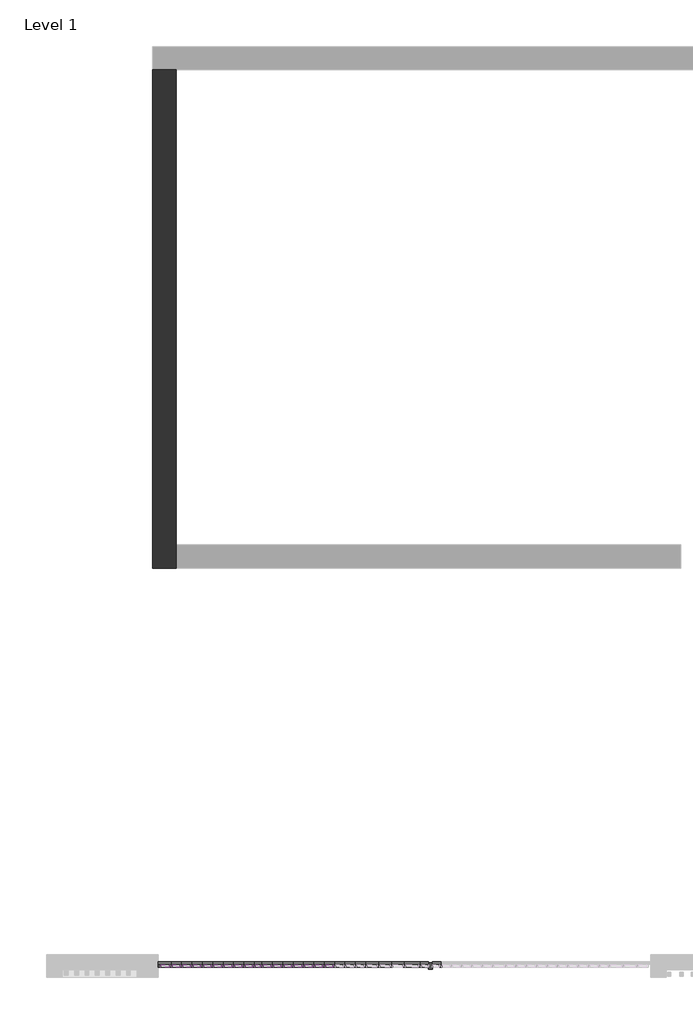
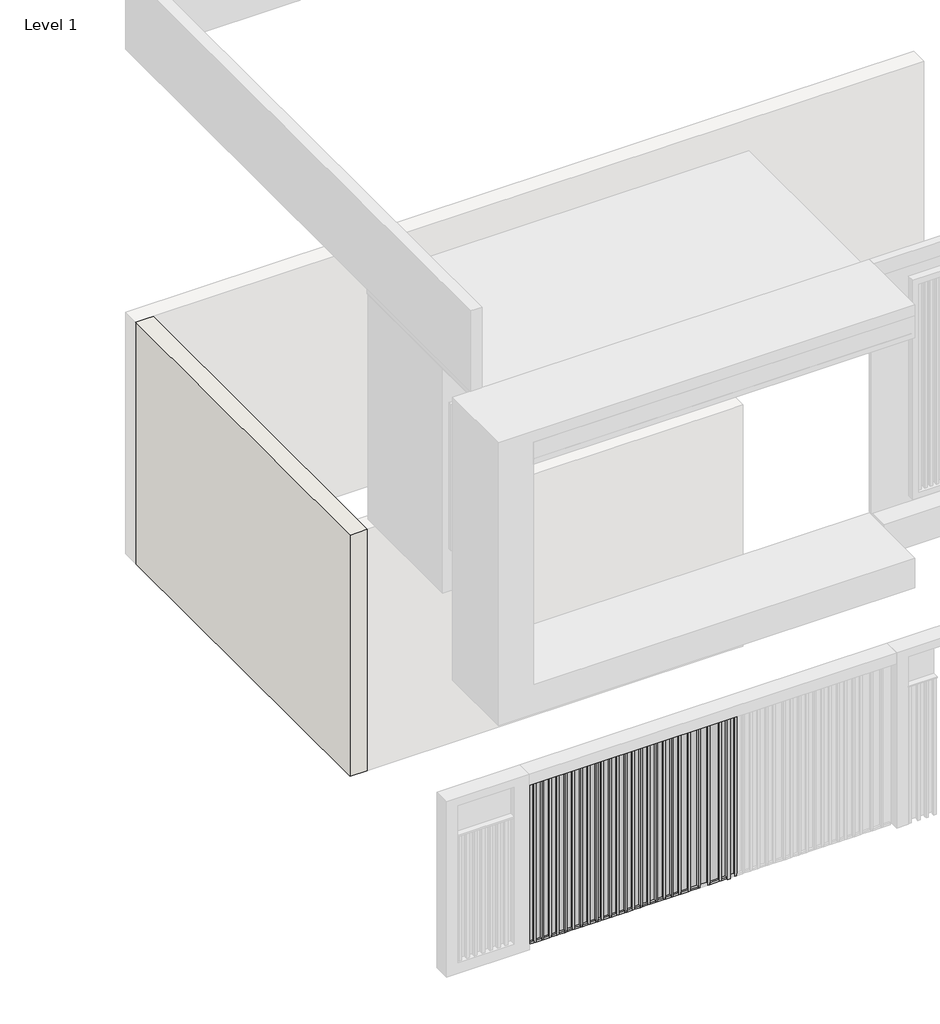
# One storey, part 1 of 2: 68 members, 26 plates, 1 wall.
"""IFC4 building model written with IfcOpenShell, lengths in millimetres."""

from ifc_helpers import new_model, si_unit, origin, place, context, project, spatial, faceted_brep, transform, mapped, element, save
from components import member_fbb4b654, member_f9b59f6e, member_4ec4fa50, member_b36ee676, member_838ad8ec, member_06b3b9e2, member_d2c643f7, member_7046656e, member_7a5d2db7, system_panel_glazed_24bd3515, system_panel_glazed_eef689be, system_panel_glazed_28c5fff6, system_panel_glazed_1ebf9f1f, system_panel_glazed_de0ba7c8

model = new_model("IFC4")

# Units and contexts
model_context = context("Model", 3, world=origin())
ifc_project = project(units=[si_unit("LENGTHUNIT", "METRE", prefix="MILLI")], contexts=[model_context])

# Site, building, storey
site = spatial("IfcSite", under=ifc_project)
building = spatial("IfcBuilding", under=site)
storey = spatial("IfcBuildingStorey", under=building, Name="Level 1", Elevation=-304.8)

# Members
placement = place(None, origin())
member_shape = member_fbb4b654(model_context)
element("IfcMember", 1, ObjectType="Rectangular Mullion : 1\" Square", at=placement, inside=storey, context=model_context, shape_type="MappedRepresentation", body=[
    mapped(member_shape, transform((-9782.3379854, -6958.7165974, -304.8), x_axis=(0.0, 0.0, -1.0), y_axis=(0.0, -1.0, 0.0), z_axis=(-1.0, 0.0, 0.0))),
])
member_2_shape = member_f9b59f6e(model_context)
element("IfcMember", 2, ObjectType="Rectangular Mullion : 1\" Square", at=placement, inside=storey, context=model_context, shape_type="MappedRepresentation", body=[
    mapped(member_2_shape, transform((-7394.7379854, -6958.7165974, -304.8), x_axis=(1.0, 0.0, 0.0), y_axis=(0.0, -1.0, 0.0), z_axis=(0.0, 0.0, -1.0))),
])
element("IfcMember", 3, ObjectType="Rectangular Mullion : 1\" Square", at=placement, inside=storey, context=model_context, shape_type="MappedRepresentation", body=[
    mapped(member_2_shape, transform((-7242.3379854, -6958.7165974, -304.8), x_axis=(1.0, 0.0, 0.0), y_axis=(0.0, -1.0, 0.0), z_axis=(0.0, 0.0, -1.0))),
])
element("IfcMember", 4, ObjectType="Rectangular Mullion : 1\" Square", at=placement, inside=storey, context=model_context, shape_type="MappedRepresentation", body=[
    mapped(member_2_shape, transform((-9680.7379854, -6958.7165974, -304.8), x_axis=(1.0, 0.0, 0.0), y_axis=(0.0, -1.0, 0.0), z_axis=(0.0, 0.0, -1.0))),
])
element("IfcMember", 5, ObjectType="Rectangular Mullion : 1\" Square", at=placement, inside=storey, context=model_context, shape_type="MappedRepresentation", body=[
    mapped(member_2_shape, transform((-9579.1379854, -6958.7165974, -304.8), x_axis=(1.0, 0.0, 0.0), y_axis=(0.0, -1.0, 0.0), z_axis=(0.0, 0.0, -1.0))),
])
element("IfcMember", 6, ObjectType="Rectangular Mullion : 1\" Square", at=placement, inside=storey, context=model_context, shape_type="MappedRepresentation", body=[
    mapped(member_2_shape, transform((-9477.5379854, -6958.7165974, -304.8), x_axis=(1.0, 0.0, 0.0), y_axis=(0.0, -1.0, 0.0), z_axis=(0.0, 0.0, -1.0))),
])
element("IfcMember", 7, ObjectType="Rectangular Mullion : 1\" Square", at=placement, inside=storey, context=model_context, shape_type="MappedRepresentation", body=[
    mapped(member_2_shape, transform((-9375.9379854, -6958.7165974, -304.8), x_axis=(1.0, 0.0, 0.0), y_axis=(0.0, -1.0, 0.0), z_axis=(0.0, 0.0, -1.0))),
])
element("IfcMember", 8, ObjectType="Rectangular Mullion : 1\" Square", at=placement, inside=storey, context=model_context, shape_type="MappedRepresentation", body=[
    mapped(member_2_shape, transform((-9274.3379854, -6958.7165974, -304.8), x_axis=(1.0, 0.0, 0.0), y_axis=(0.0, -1.0, 0.0), z_axis=(0.0, 0.0, -1.0))),
])
element("IfcMember", 9, ObjectType="Rectangular Mullion : 1\" Square", at=placement, inside=storey, context=model_context, shape_type="MappedRepresentation", body=[
    mapped(member_2_shape, transform((-9172.7379854, -6958.7165974, -304.8), x_axis=(1.0, 0.0, 0.0), y_axis=(0.0, -1.0, 0.0), z_axis=(0.0, 0.0, -1.0))),
])
element("IfcMember", 10, ObjectType="Rectangular Mullion : 1\" Square", at=placement, inside=storey, context=model_context, shape_type="MappedRepresentation", body=[
    mapped(member_2_shape, transform((-9071.1379854, -6958.7165974, -304.8), x_axis=(1.0, 0.0, 0.0), y_axis=(0.0, -1.0, 0.0), z_axis=(0.0, 0.0, -1.0))),
])
element("IfcMember", 11, ObjectType="Rectangular Mullion : 1\" Square", at=placement, inside=storey, context=model_context, shape_type="MappedRepresentation", body=[
    mapped(member_2_shape, transform((-8969.5379854, -6958.7165974, -304.8), x_axis=(1.0, 0.0, 0.0), y_axis=(0.0, -1.0, 0.0), z_axis=(0.0, 0.0, -1.0))),
])
element("IfcMember", 12, ObjectType="Rectangular Mullion : 1\" Square", at=placement, inside=storey, context=model_context, shape_type="MappedRepresentation", body=[
    mapped(member_2_shape, transform((-8867.9379854, -6958.7165974, -304.8), x_axis=(1.0, 0.0, 0.0), y_axis=(0.0, -1.0, 0.0), z_axis=(0.0, 0.0, -1.0))),
])
element("IfcMember", 13, ObjectType="Rectangular Mullion : 1\" Square", at=placement, inside=storey, context=model_context, shape_type="MappedRepresentation", body=[
    mapped(member_2_shape, transform((-8791.7379854, -6958.7165974, -304.8), x_axis=(1.0, 0.0, 0.0), y_axis=(0.0, -1.0, 0.0), z_axis=(0.0, 0.0, -1.0))),
])
element("IfcMember", 14, ObjectType="Rectangular Mullion : 1\" Square", at=placement, inside=storey, context=model_context, shape_type="MappedRepresentation", body=[
    mapped(member_2_shape, transform((-8690.1379854, -6958.7165974, -304.8), x_axis=(1.0, 0.0, 0.0), y_axis=(0.0, -1.0, 0.0), z_axis=(0.0, 0.0, -1.0))),
])
element("IfcMember", 15, ObjectType="Rectangular Mullion : 1\" Square", at=placement, inside=storey, context=model_context, shape_type="MappedRepresentation", body=[
    mapped(member_2_shape, transform((-8588.5379854, -6958.7165974, -304.8), x_axis=(1.0, 0.0, 0.0), y_axis=(0.0, -1.0, 0.0), z_axis=(0.0, 0.0, -1.0))),
])
element("IfcMember", 16, ObjectType="Rectangular Mullion : 1\" Square", at=placement, inside=storey, context=model_context, shape_type="MappedRepresentation", body=[
    mapped(member_2_shape, transform((-8486.9379854, -6958.7165974, -304.8), x_axis=(1.0, 0.0, 0.0), y_axis=(0.0, -1.0, 0.0), z_axis=(0.0, 0.0, -1.0))),
])
element("IfcMember", 17, ObjectType="Rectangular Mullion : 1\" Square", at=placement, inside=storey, context=model_context, shape_type="MappedRepresentation", body=[
    mapped(member_2_shape, transform((-8385.3379854, -6958.7165974, -304.8), x_axis=(1.0, 0.0, 0.0), y_axis=(0.0, -1.0, 0.0), z_axis=(0.0, 0.0, -1.0))),
])
element("IfcMember", 18, ObjectType="Rectangular Mullion : 1\" Square", at=placement, inside=storey, context=model_context, shape_type="MappedRepresentation", body=[
    mapped(member_2_shape, transform((-8283.7379854, -6958.7165974, -304.8), x_axis=(1.0, 0.0, 0.0), y_axis=(0.0, -1.0, 0.0), z_axis=(0.0, 0.0, -1.0))),
])
element("IfcMember", 19, ObjectType="Rectangular Mullion : 1\" Square", at=placement, inside=storey, context=model_context, shape_type="MappedRepresentation", body=[
    mapped(member_2_shape, transform((-8182.1379854, -6958.7165974, -304.8), x_axis=(1.0, 0.0, 0.0), y_axis=(0.0, -1.0, 0.0), z_axis=(0.0, 0.0, -1.0))),
])
element("IfcMember", 20, ObjectType="Rectangular Mullion : 1\" Square", at=placement, inside=storey, context=model_context, shape_type="MappedRepresentation", body=[
    mapped(member_2_shape, transform((-8080.5379854, -6958.7165974, -304.8), x_axis=(1.0, 0.0, 0.0), y_axis=(0.0, -1.0, 0.0), z_axis=(0.0, 0.0, -1.0))),
])
element("IfcMember", 21, ObjectType="Rectangular Mullion : 1\" Square", at=placement, inside=storey, context=model_context, shape_type="MappedRepresentation", body=[
    mapped(member_2_shape, transform((-7978.9379854, -6958.7165974, -304.8), x_axis=(1.0, 0.0, 0.0), y_axis=(0.0, -1.0, 0.0), z_axis=(0.0, 0.0, -1.0))),
])
element("IfcMember", 22, ObjectType="Rectangular Mullion : 1\" Square", at=placement, inside=storey, context=model_context, shape_type="MappedRepresentation", body=[
    mapped(member_2_shape, transform((-7877.3379854, -6958.7165974, -304.8), x_axis=(1.0, 0.0, 0.0), y_axis=(0.0, -1.0, 0.0), z_axis=(0.0, 0.0, -1.0))),
])
element("IfcMember", 23, ObjectType="Rectangular Mullion : 1\" Square", at=placement, inside=storey, context=model_context, shape_type="MappedRepresentation", body=[
    mapped(member_2_shape, transform((-7775.7379854, -6958.7165974, -304.8), x_axis=(1.0, 0.0, 0.0), y_axis=(0.0, -1.0, 0.0), z_axis=(0.0, 0.0, -1.0))),
])
element("IfcMember", 24, ObjectType="Rectangular Mullion : 1\" Square", at=placement, inside=storey, context=model_context, shape_type="MappedRepresentation", body=[
    mapped(member_2_shape, transform((-7648.7379854, -6958.7165974, -304.8), x_axis=(1.0, 0.0, 0.0), y_axis=(0.0, -1.0, 0.0), z_axis=(0.0, 0.0, -1.0))),
])
element("IfcMember", 25, ObjectType="Rectangular Mullion : 1\" Square", at=placement, inside=storey, context=model_context, shape_type="MappedRepresentation", body=[
    mapped(member_2_shape, transform((-7521.7379854, -6958.7165974, -304.8), x_axis=(1.0, 0.0, 0.0), y_axis=(0.0, -1.0, 0.0), z_axis=(0.0, 0.0, -1.0))),
])
element("IfcMember", 26, ObjectType="Rectangular Mullion : 1\" Square", at=placement, inside=storey, context=model_context, shape_type="MappedRepresentation", body=[
    mapped(member_2_shape, transform((-7039.1379854, -6958.7165974, -304.8), x_axis=(1.0, 0.0, 0.0), y_axis=(0.0, -1.0, 0.0), z_axis=(0.0, 0.0, -1.0))),
])
member_3_shape = member_4ec4fa50(model_context)
element("IfcMember", 27, ObjectType="Rectangular Mullion : 1\" Square", at=placement, inside=storey, context=model_context, shape_type="MappedRepresentation", body=[
    mapped(member_3_shape, transform((-7382.0379854, -6958.7165974, -304.8), x_axis=(0.0, 0.0, -1.0), y_axis=(0.0, -1.0, 0.0), z_axis=(-1.0, 0.0, 0.0))),
])
member_4_shape = member_b36ee676(model_context)
element("IfcMember", 28, ObjectType="Rectangular Mullion : 1\" Square", at=placement, inside=storey, context=model_context, shape_type="MappedRepresentation", body=[
    mapped(member_4_shape, transform((-7229.6379854, -6958.7165974, -304.8), x_axis=(0.0, 0.0, -1.0), y_axis=(0.0, -1.0, 0.0), z_axis=(-1.0, 0.0, 0.0))),
])
member_5_shape = member_838ad8ec(model_context)
element("IfcMember", 29, ObjectType="Rectangular Mullion : 1\" Square", at=placement, inside=storey, context=model_context, shape_type="MappedRepresentation", body=[
    mapped(member_5_shape, transform((-9668.0379854, -6958.7165974, -304.8), x_axis=(0.0, 0.0, -1.0), y_axis=(0.0, -1.0, 0.0), z_axis=(-1.0, 0.0, 0.0))),
])
element("IfcMember", 30, ObjectType="Rectangular Mullion : 1\" Square", at=placement, inside=storey, context=model_context, shape_type="MappedRepresentation", body=[
    mapped(member_5_shape, transform((-9566.4379854, -6958.7165974, -304.8), x_axis=(0.0, 0.0, -1.0), y_axis=(0.0, -1.0, 0.0), z_axis=(-1.0, 0.0, 0.0))),
])
element("IfcMember", 31, ObjectType="Rectangular Mullion : 1\" Square", at=placement, inside=storey, context=model_context, shape_type="MappedRepresentation", body=[
    mapped(member_5_shape, transform((-9464.8379854, -6958.7165974, -304.8), x_axis=(0.0, 0.0, -1.0), y_axis=(0.0, -1.0, 0.0), z_axis=(-1.0, 0.0, 0.0))),
])
element("IfcMember", 32, ObjectType="Rectangular Mullion : 1\" Square", at=placement, inside=storey, context=model_context, shape_type="MappedRepresentation", body=[
    mapped(member_5_shape, transform((-9363.2379854, -6958.7165974, -304.8), x_axis=(0.0, 0.0, -1.0), y_axis=(0.0, -1.0, 0.0), z_axis=(-1.0, 0.0, 0.0))),
])
element("IfcMember", 33, ObjectType="Rectangular Mullion : 1\" Square", at=placement, inside=storey, context=model_context, shape_type="MappedRepresentation", body=[
    mapped(member_5_shape, transform((-9261.6379854, -6958.7165974, -304.8), x_axis=(0.0, 0.0, -1.0), y_axis=(0.0, -1.0, 0.0), z_axis=(-1.0, 0.0, 0.0))),
])
element("IfcMember", 34, ObjectType="Rectangular Mullion : 1\" Square", at=placement, inside=storey, context=model_context, shape_type="MappedRepresentation", body=[
    mapped(member_5_shape, transform((-9160.0379854, -6958.7165974, -304.8), x_axis=(0.0, 0.0, -1.0), y_axis=(0.0, -1.0, 0.0), z_axis=(-1.0, 0.0, 0.0))),
])
element("IfcMember", 35, ObjectType="Rectangular Mullion : 1\" Square", at=placement, inside=storey, context=model_context, shape_type="MappedRepresentation", body=[
    mapped(member_5_shape, transform((-9058.4379854, -6958.7165974, -304.8), x_axis=(0.0, 0.0, -1.0), y_axis=(0.0, -1.0, 0.0), z_axis=(-1.0, 0.0, 0.0))),
])
element("IfcMember", 36, ObjectType="Rectangular Mullion : 1\" Square", at=placement, inside=storey, context=model_context, shape_type="MappedRepresentation", body=[
    mapped(member_5_shape, transform((-8956.8379854, -6958.7165974, -304.8), x_axis=(0.0, 0.0, -1.0), y_axis=(0.0, -1.0, 0.0), z_axis=(-1.0, 0.0, 0.0))),
])
element("IfcMember", 37, ObjectType="Rectangular Mullion : 1\" Square", at=placement, inside=storey, context=model_context, shape_type="MappedRepresentation", body=[
    mapped(member_5_shape, transform((-8779.0379854, -6958.7165974, -304.8), x_axis=(0.0, 0.0, -1.0), y_axis=(0.0, -1.0, 0.0), z_axis=(-1.0, 0.0, 0.0))),
])
element("IfcMember", 38, ObjectType="Rectangular Mullion : 1\" Square", at=placement, inside=storey, context=model_context, shape_type="MappedRepresentation", body=[
    mapped(member_5_shape, transform((-8677.4379854, -6958.7165974, -304.8), x_axis=(0.0, 0.0, -1.0), y_axis=(0.0, -1.0, 0.0), z_axis=(-1.0, 0.0, 0.0))),
])
element("IfcMember", 39, ObjectType="Rectangular Mullion : 1\" Square", at=placement, inside=storey, context=model_context, shape_type="MappedRepresentation", body=[
    mapped(member_5_shape, transform((-8575.8379854, -6958.7165974, -304.8), x_axis=(0.0, 0.0, -1.0), y_axis=(0.0, -1.0, 0.0), z_axis=(-1.0, 0.0, 0.0))),
])
element("IfcMember", 40, ObjectType="Rectangular Mullion : 1\" Square", at=placement, inside=storey, context=model_context, shape_type="MappedRepresentation", body=[
    mapped(member_5_shape, transform((-8474.2379854, -6958.7165974, -304.8), x_axis=(0.0, 0.0, -1.0), y_axis=(0.0, -1.0, 0.0), z_axis=(-1.0, 0.0, 0.0))),
])
element("IfcMember", 41, ObjectType="Rectangular Mullion : 1\" Square", at=placement, inside=storey, context=model_context, shape_type="MappedRepresentation", body=[
    mapped(member_5_shape, transform((-8372.6379854, -6958.7165974, -304.8), x_axis=(0.0, 0.0, -1.0), y_axis=(0.0, -1.0, 0.0), z_axis=(-1.0, 0.0, 0.0))),
])
element("IfcMember", 42, ObjectType="Rectangular Mullion : 1\" Square", at=placement, inside=storey, context=model_context, shape_type="MappedRepresentation", body=[
    mapped(member_5_shape, transform((-8271.0379854, -6958.7165974, -304.8), x_axis=(0.0, 0.0, -1.0), y_axis=(0.0, -1.0, 0.0), z_axis=(-1.0, 0.0, 0.0))),
])
element("IfcMember", 43, ObjectType="Rectangular Mullion : 1\" Square", at=placement, inside=storey, context=model_context, shape_type="MappedRepresentation", body=[
    mapped(member_5_shape, transform((-8169.4379854, -6958.7165974, -304.8), x_axis=(0.0, 0.0, -1.0), y_axis=(0.0, -1.0, 0.0), z_axis=(-1.0, 0.0, 0.0))),
])
element("IfcMember", 44, ObjectType="Rectangular Mullion : 1\" Square", at=placement, inside=storey, context=model_context, shape_type="MappedRepresentation", body=[
    mapped(member_5_shape, transform((-8067.8379854, -6958.7165974, -304.8), x_axis=(0.0, 0.0, -1.0), y_axis=(0.0, -1.0, 0.0), z_axis=(-1.0, 0.0, 0.0))),
])
element("IfcMember", 45, ObjectType="Rectangular Mullion : 1\" Square", at=placement, inside=storey, context=model_context, shape_type="MappedRepresentation", body=[
    mapped(member_5_shape, transform((-7966.2379854, -6958.7165974, -304.8), x_axis=(0.0, 0.0, -1.0), y_axis=(0.0, -1.0, 0.0), z_axis=(-1.0, 0.0, 0.0))),
])
element("IfcMember", 46, ObjectType="Rectangular Mullion : 1\" Square", at=placement, inside=storey, context=model_context, shape_type="MappedRepresentation", body=[
    mapped(member_5_shape, transform((-7864.6379854, -6958.7165974, -304.8), x_axis=(0.0, 0.0, -1.0), y_axis=(0.0, -1.0, 0.0), z_axis=(-1.0, 0.0, 0.0))),
])
member_6_shape = member_06b3b9e2(model_context)
element("IfcMember", 47, ObjectType="Rectangular Mullion : 1\" Square", at=placement, inside=storey, context=model_context, shape_type="MappedRepresentation", body=[
    mapped(member_6_shape, transform((-8855.2379854, -6958.7165974, -304.8), x_axis=(0.0, 0.0, -1.0), y_axis=(0.0, -1.0, 0.0), z_axis=(-1.0, 0.0, 0.0))),
])
member_7_shape = member_d2c643f7(model_context)
element("IfcMember", 48, ObjectType="Rectangular Mullion : 1\" Square", at=placement, inside=storey, context=model_context, shape_type="MappedRepresentation", body=[
    mapped(member_7_shape, transform((-7763.0379854, -6958.7165974, -304.8), x_axis=(0.0, 0.0, -1.0), y_axis=(0.0, -1.0, 0.0), z_axis=(-1.0, 0.0, 0.0))),
])
element("IfcMember", 49, ObjectType="Rectangular Mullion : 1\" Square", at=placement, inside=storey, context=model_context, shape_type="MappedRepresentation", body=[
    mapped(member_7_shape, transform((-7636.0379854, -6958.7165974, -304.8), x_axis=(0.0, 0.0, -1.0), y_axis=(0.0, -1.0, 0.0), z_axis=(-1.0, 0.0, 0.0))),
])
element("IfcMember", 50, ObjectType="Rectangular Mullion : 1\" Square", at=placement, inside=storey, context=model_context, shape_type="MappedRepresentation", body=[
    mapped(member_shape, transform((-9693.4379854, -6958.7165974, 1982.7875), x_axis=(0.0, 0.0, 1.0), y_axis=(0.0, -1.0, 0.0), z_axis=(1.0, 0.0, 0.0))),
])
element("IfcMember", 51, ObjectType="Rectangular Mullion : 1\" Square", at=placement, inside=storey, context=model_context, shape_type="MappedRepresentation", body=[
    mapped(member_5_shape, transform((-9591.8379854, -6958.7165974, 1982.7875), x_axis=(0.0, 0.0, 1.0), y_axis=(0.0, -1.0, 0.0), z_axis=(1.0, 0.0, 0.0))),
])
element("IfcMember", 52, ObjectType="Rectangular Mullion : 1\" Square", at=placement, inside=storey, context=model_context, shape_type="MappedRepresentation", body=[
    mapped(member_5_shape, transform((-9490.2379854, -6958.7165974, 1982.7875), x_axis=(0.0, 0.0, 1.0), y_axis=(0.0, -1.0, 0.0), z_axis=(1.0, 0.0, 0.0))),
])
element("IfcMember", 53, ObjectType="Rectangular Mullion : 1\" Square", at=placement, inside=storey, context=model_context, shape_type="MappedRepresentation", body=[
    mapped(member_5_shape, transform((-9388.6379854, -6958.7165974, 1982.7875), x_axis=(0.0, 0.0, 1.0), y_axis=(0.0, -1.0, 0.0), z_axis=(1.0, 0.0, 0.0))),
])
element("IfcMember", 54, ObjectType="Rectangular Mullion : 1\" Square", at=placement, inside=storey, context=model_context, shape_type="MappedRepresentation", body=[
    mapped(member_5_shape, transform((-9287.0379854, -6958.7165974, 1982.7875), x_axis=(0.0, 0.0, 1.0), y_axis=(0.0, -1.0, 0.0), z_axis=(1.0, 0.0, 0.0))),
])
element("IfcMember", 55, ObjectType="Rectangular Mullion : 1\" Square", at=placement, inside=storey, context=model_context, shape_type="MappedRepresentation", body=[
    mapped(member_5_shape, transform((-9185.4379854, -6958.7165974, 1982.7875), x_axis=(0.0, 0.0, 1.0), y_axis=(0.0, -1.0, 0.0), z_axis=(1.0, 0.0, 0.0))),
])
element("IfcMember", 56, ObjectType="Rectangular Mullion : 1\" Square", at=placement, inside=storey, context=model_context, shape_type="MappedRepresentation", body=[
    mapped(member_5_shape, transform((-9083.8379854, -6958.7165974, 1982.7875), x_axis=(0.0, 0.0, 1.0), y_axis=(0.0, -1.0, 0.0), z_axis=(1.0, 0.0, 0.0))),
])
element("IfcMember", 57, ObjectType="Rectangular Mullion : 1\" Square", at=placement, inside=storey, context=model_context, shape_type="MappedRepresentation", body=[
    mapped(member_5_shape, transform((-8982.2379854, -6958.7165974, 1982.7875), x_axis=(0.0, 0.0, 1.0), y_axis=(0.0, -1.0, 0.0), z_axis=(1.0, 0.0, 0.0))),
])
element("IfcMember", 58, ObjectType="Rectangular Mullion : 1\" Square", at=placement, inside=storey, context=model_context, shape_type="MappedRepresentation", body=[
    mapped(member_5_shape, transform((-8880.6379854, -6958.7165974, 1982.7875), x_axis=(0.0, 0.0, 1.0), y_axis=(0.0, -1.0, 0.0), z_axis=(1.0, 0.0, 0.0))),
])
element("IfcMember", 59, ObjectType="Rectangular Mullion : 1\" Square", at=placement, inside=storey, context=model_context, shape_type="MappedRepresentation", body=[
    mapped(member_5_shape, transform((-8702.8379854, -6958.7165974, 1982.7875), x_axis=(0.0, 0.0, 1.0), y_axis=(0.0, -1.0, 0.0), z_axis=(1.0, 0.0, 0.0))),
])
element("IfcMember", 60, ObjectType="Rectangular Mullion : 1\" Square", at=placement, inside=storey, context=model_context, shape_type="MappedRepresentation", body=[
    mapped(member_5_shape, transform((-8601.2379854, -6958.7165974, 1982.7875), x_axis=(0.0, 0.0, 1.0), y_axis=(0.0, -1.0, 0.0), z_axis=(1.0, 0.0, 0.0))),
])
element("IfcMember", 61, ObjectType="Rectangular Mullion : 1\" Square", at=placement, inside=storey, context=model_context, shape_type="MappedRepresentation", body=[
    mapped(member_5_shape, transform((-8499.6379854, -6958.7165974, 1982.7875), x_axis=(0.0, 0.0, 1.0), y_axis=(0.0, -1.0, 0.0), z_axis=(1.0, 0.0, 0.0))),
])
element("IfcMember", 62, ObjectType="Rectangular Mullion : 1\" Square", at=placement, inside=storey, context=model_context, shape_type="MappedRepresentation", body=[
    mapped(member_5_shape, transform((-8398.0379854, -6958.7165974, 1982.7875), x_axis=(0.0, 0.0, 1.0), y_axis=(0.0, -1.0, 0.0), z_axis=(1.0, 0.0, 0.0))),
])
element("IfcMember", 63, ObjectType="Rectangular Mullion : 1\" Square", at=placement, inside=storey, context=model_context, shape_type="MappedRepresentation", body=[
    mapped(member_5_shape, transform((-8296.4379854, -6958.7165974, 1982.7875), x_axis=(0.0, 0.0, 1.0), y_axis=(0.0, -1.0, 0.0), z_axis=(1.0, 0.0, 0.0))),
])
element("IfcMember", 64, ObjectType="Rectangular Mullion : 1\" Square", at=placement, inside=storey, context=model_context, shape_type="MappedRepresentation", body=[
    mapped(member_5_shape, transform((-8194.8379854, -6958.7165974, 1982.7875), x_axis=(0.0, 0.0, 1.0), y_axis=(0.0, -1.0, 0.0), z_axis=(1.0, 0.0, 0.0))),
])
element("IfcMember", 65, ObjectType="Rectangular Mullion : 1\" Square", at=placement, inside=storey, context=model_context, shape_type="MappedRepresentation", body=[
    mapped(member_5_shape, transform((-8093.2379854, -6958.7165974, 1982.7875), x_axis=(0.0, 0.0, 1.0), y_axis=(0.0, -1.0, 0.0), z_axis=(1.0, 0.0, 0.0))),
])
element("IfcMember", 66, ObjectType="Rectangular Mullion : 1\" Square", at=placement, inside=storey, context=model_context, shape_type="MappedRepresentation", body=[
    mapped(member_6_shape, transform((-8804.4379854, -6958.7165974, 1982.7875), x_axis=(0.0, 0.0, 1.0), y_axis=(0.0, -1.0, 0.0), z_axis=(1.0, 0.0, 0.0))),
])
member_8_shape = member_7046656e(model_context)
element("IfcMember", 67, ObjectType="Rectangular Mullion : 1\" Square", at=placement, inside=storey, context=model_context, shape_type="MappedRepresentation", body=[
    mapped(member_8_shape, transform((-9807.7379854, -6958.7165974, 1982.7875), x_axis=(-1.0, 0.0, 0.0), y_axis=(0.0, -1.0, 0.0), z_axis=(0.0, 0.0, 1.0))),
])
member_9_shape = member_7a5d2db7(model_context)
element("IfcMember", 68, ObjectType="Rectangular Mullion : 1.5\" x 2.5\" rectangular", at=placement, inside=storey, context=model_context, shape_type="MappedRepresentation", body=[
    mapped(member_9_shape, transform((-7140.7379854, -6958.7165974, -304.8), x_axis=(1.0, 0.0, 0.0), y_axis=(0.0, -1.0, 0.0), z_axis=(0.0, 0.0, -1.0))),
])

# Plates
system_panel_glazed_shape = system_panel_glazed_24bd3515(model_context)
element("IfcPlate", 69, ObjectType="System Panel : Glazed", at=placement, inside=storey, context=model_context, shape_type="MappedRepresentation", body=[
    mapped(system_panel_glazed_shape, transform((-7318.5379854, -6958.7165974, -304.8), x_axis=(1.0, 0.0, 0.0), y_axis=(0.0, 1.0, 0.0), z_axis=(0.0, 0.0, 1.0))),
])
system_panel_glazed_2_shape = system_panel_glazed_eef689be(model_context)
element("IfcPlate", 70, ObjectType="System Panel : Glazed", at=placement, inside=storey, context=model_context, shape_type="MappedRepresentation", body=[
    mapped(system_panel_glazed_2_shape, transform((-9744.2379854, -6958.7165974, -304.8), x_axis=(1.0, 0.0, 0.0), y_axis=(0.0, 1.0, 0.0), z_axis=(0.0, 0.0, 1.0))),
])
element("IfcPlate", 71, ObjectType="System Panel : Glazed", at=placement, inside=storey, context=model_context, shape_type="MappedRepresentation", body=[
    mapped(system_panel_glazed_2_shape, transform((-7712.2379854, -6958.7165974, -304.8), x_axis=(1.0, 0.0, 0.0), y_axis=(0.0, 1.0, 0.0), z_axis=(0.0, 0.0, 1.0))),
])
element("IfcPlate", 72, ObjectType="System Panel : Glazed", at=placement, inside=storey, context=model_context, shape_type="MappedRepresentation", body=[
    mapped(system_panel_glazed_2_shape, transform((-7585.2379854, -6958.7165974, -304.8), x_axis=(1.0, 0.0, 0.0), y_axis=(0.0, 1.0, 0.0), z_axis=(0.0, 0.0, 1.0))),
])
element("IfcPlate", 73, ObjectType="System Panel : Glazed", at=placement, inside=storey, context=model_context, shape_type="MappedRepresentation", body=[
    mapped(system_panel_glazed_2_shape, transform((-7458.2379854, -6958.7165974, -304.8), x_axis=(1.0, 0.0, 0.0), y_axis=(0.0, 1.0, 0.0), z_axis=(0.0, 0.0, 1.0))),
])
system_panel_glazed_3_shape = system_panel_glazed_28c5fff6(model_context)
element("IfcPlate", 74, ObjectType="System Panel : Glazed", at=placement, inside=storey, context=model_context, shape_type="MappedRepresentation", body=[
    mapped(system_panel_glazed_3_shape, transform((-9629.9379854, -6958.7165974, -304.8), x_axis=(1.0, 0.0, 0.0), y_axis=(0.0, 1.0, 0.0), z_axis=(0.0, 0.0, 1.0))),
])
element("IfcPlate", 75, ObjectType="System Panel : Glazed", at=placement, inside=storey, context=model_context, shape_type="MappedRepresentation", body=[
    mapped(system_panel_glazed_3_shape, transform((-9528.3379854, -6958.7165974, -304.8), x_axis=(1.0, 0.0, 0.0), y_axis=(0.0, 1.0, 0.0), z_axis=(0.0, 0.0, 1.0))),
])
element("IfcPlate", 76, ObjectType="System Panel : Glazed", at=placement, inside=storey, context=model_context, shape_type="MappedRepresentation", body=[
    mapped(system_panel_glazed_3_shape, transform((-9426.7379854, -6958.7165974, -304.8), x_axis=(1.0, 0.0, 0.0), y_axis=(0.0, 1.0, 0.0), z_axis=(0.0, 0.0, 1.0))),
])
element("IfcPlate", 77, ObjectType="System Panel : Glazed", at=placement, inside=storey, context=model_context, shape_type="MappedRepresentation", body=[
    mapped(system_panel_glazed_3_shape, transform((-9325.1379854, -6958.7165974, -304.8), x_axis=(1.0, 0.0, 0.0), y_axis=(0.0, 1.0, 0.0), z_axis=(0.0, 0.0, 1.0))),
])
element("IfcPlate", 78, ObjectType="System Panel : Glazed", at=placement, inside=storey, context=model_context, shape_type="MappedRepresentation", body=[
    mapped(system_panel_glazed_3_shape, transform((-9223.5379854, -6958.7165974, -304.8), x_axis=(1.0, 0.0, 0.0), y_axis=(0.0, 1.0, 0.0), z_axis=(0.0, 0.0, 1.0))),
])
element("IfcPlate", 79, ObjectType="System Panel : Glazed", at=placement, inside=storey, context=model_context, shape_type="MappedRepresentation", body=[
    mapped(system_panel_glazed_3_shape, transform((-9121.9379854, -6958.7165974, -304.8), x_axis=(1.0, 0.0, 0.0), y_axis=(0.0, 1.0, 0.0), z_axis=(0.0, 0.0, 1.0))),
])
element("IfcPlate", 80, ObjectType="System Panel : Glazed", at=placement, inside=storey, context=model_context, shape_type="MappedRepresentation", body=[
    mapped(system_panel_glazed_3_shape, transform((-9020.3379854, -6958.7165974, -304.8), x_axis=(1.0, 0.0, 0.0), y_axis=(0.0, 1.0, 0.0), z_axis=(0.0, 0.0, 1.0))),
])
element("IfcPlate", 81, ObjectType="System Panel : Glazed", at=placement, inside=storey, context=model_context, shape_type="MappedRepresentation", body=[
    mapped(system_panel_glazed_3_shape, transform((-8918.7379854, -6958.7165974, -304.8), x_axis=(1.0, 0.0, 0.0), y_axis=(0.0, 1.0, 0.0), z_axis=(0.0, 0.0, 1.0))),
])
element("IfcPlate", 82, ObjectType="System Panel : Glazed", at=placement, inside=storey, context=model_context, shape_type="MappedRepresentation", body=[
    mapped(system_panel_glazed_3_shape, transform((-8740.9379854, -6958.7165974, -304.8), x_axis=(1.0, 0.0, 0.0), y_axis=(0.0, 1.0, 0.0), z_axis=(0.0, 0.0, 1.0))),
])
element("IfcPlate", 83, ObjectType="System Panel : Glazed", at=placement, inside=storey, context=model_context, shape_type="MappedRepresentation", body=[
    mapped(system_panel_glazed_3_shape, transform((-8639.3379854, -6958.7165974, -304.8), x_axis=(1.0, 0.0, 0.0), y_axis=(0.0, 1.0, 0.0), z_axis=(0.0, 0.0, 1.0))),
])
element("IfcPlate", 84, ObjectType="System Panel : Glazed", at=placement, inside=storey, context=model_context, shape_type="MappedRepresentation", body=[
    mapped(system_panel_glazed_3_shape, transform((-8537.7379854, -6958.7165974, -304.8), x_axis=(1.0, 0.0, 0.0), y_axis=(0.0, 1.0, 0.0), z_axis=(0.0, 0.0, 1.0))),
])
element("IfcPlate", 85, ObjectType="System Panel : Glazed", at=placement, inside=storey, context=model_context, shape_type="MappedRepresentation", body=[
    mapped(system_panel_glazed_3_shape, transform((-8436.1379854, -6958.7165974, -304.8), x_axis=(1.0, 0.0, 0.0), y_axis=(0.0, 1.0, 0.0), z_axis=(0.0, 0.0, 1.0))),
])
element("IfcPlate", 86, ObjectType="System Panel : Glazed", at=placement, inside=storey, context=model_context, shape_type="MappedRepresentation", body=[
    mapped(system_panel_glazed_3_shape, transform((-8334.5379854, -6958.7165974, -304.8), x_axis=(1.0, 0.0, 0.0), y_axis=(0.0, 1.0, 0.0), z_axis=(0.0, 0.0, 1.0))),
])
element("IfcPlate", 87, ObjectType="System Panel : Glazed", at=placement, inside=storey, context=model_context, shape_type="MappedRepresentation", body=[
    mapped(system_panel_glazed_3_shape, transform((-8232.9379854, -6958.7165974, -304.8), x_axis=(1.0, 0.0, 0.0), y_axis=(0.0, 1.0, 0.0), z_axis=(0.0, 0.0, 1.0))),
])
element("IfcPlate", 88, ObjectType="System Panel : Glazed", at=placement, inside=storey, context=model_context, shape_type="MappedRepresentation", body=[
    mapped(system_panel_glazed_3_shape, transform((-8131.3379854, -6958.7165974, -304.8), x_axis=(1.0, 0.0, 0.0), y_axis=(0.0, 1.0, 0.0), z_axis=(0.0, 0.0, 1.0))),
])
element("IfcPlate", 89, ObjectType="System Panel : Glazed", at=placement, inside=storey, context=model_context, shape_type="MappedRepresentation", body=[
    mapped(system_panel_glazed_3_shape, transform((-8029.7379854, -6958.7165974, -304.8), x_axis=(1.0, 0.0, 0.0), y_axis=(0.0, 1.0, 0.0), z_axis=(0.0, 0.0, 1.0))),
])
element("IfcPlate", 90, ObjectType="System Panel : Glazed", at=placement, inside=storey, context=model_context, shape_type="MappedRepresentation", body=[
    mapped(system_panel_glazed_3_shape, transform((-7928.1379854, -6958.7165974, -304.8), x_axis=(1.0, 0.0, 0.0), y_axis=(0.0, 1.0, 0.0), z_axis=(0.0, 0.0, 1.0))),
])
element("IfcPlate", 91, ObjectType="System Panel : Glazed", at=placement, inside=storey, context=model_context, shape_type="MappedRepresentation", body=[
    mapped(system_panel_glazed_3_shape, transform((-7826.5379854, -6958.7165974, -304.8), x_axis=(1.0, 0.0, 0.0), y_axis=(0.0, 1.0, 0.0), z_axis=(0.0, 0.0, 1.0))),
])
system_panel_glazed_4_shape = system_panel_glazed_1ebf9f1f(model_context)
element("IfcPlate", 92, ObjectType="System Panel : Glazed", at=placement, inside=storey, context=model_context, shape_type="MappedRepresentation", body=[
    mapped(system_panel_glazed_4_shape, transform((-8829.8379854, -6958.7165974, -304.8), x_axis=(1.0, 0.0, 0.0), y_axis=(0.0, 1.0, 0.0), z_axis=(0.0, 0.0, 1.0))),
])
system_panel_glazed_5_shape = system_panel_glazed_de0ba7c8(model_context)
element("IfcPlate", 93, ObjectType="System Panel : Glazed", at=placement, inside=storey, context=model_context, shape_type="MappedRepresentation", body=[
    mapped(system_panel_glazed_5_shape, transform((-7201.0629854, -6958.7165974, -304.8), x_axis=(1.0, 0.0, 0.0), y_axis=(0.0, 1.0, 0.0), z_axis=(0.0, 0.0, 1.0))),
])
element("IfcPlate", 94, ObjectType="System Panel : Glazed", at=placement, inside=storey, context=model_context, shape_type="MappedRepresentation", body=[
    mapped(system_panel_glazed_5_shape, transform((-7080.4129854, -6958.7165974, -304.8), x_axis=(1.0, 0.0, 0.0), y_axis=(0.0, 1.0, 0.0), z_axis=(0.0, 0.0, 1.0))),
])

# Wall
element("IfcWall", 95, ObjectType="9\" wall", at=placement, inside=storey, context=model_context, shape_type="Brep", body=[
    faceted_brep([(-9629.9379854, -3063.2506821, -304.8), (-9629.9379854, -2834.6506821, -304.8), (-9629.9379854, 1813.5493179, -304.8), (-9629.9379854, 1813.5493179, 3048.0), (-9629.9379854, -2834.6506821, 3048.0), (-9629.9379854, -3063.2506821, 3048.0), (-9858.5379854, -3063.2506821, -304.8), (-9858.5379854, -3063.2506821, 3048.0), (-9858.5379854, 1813.5493179, 3048.0), (-9858.5379854, 1813.5493179, -304.8)], [[[0, 1, 2, 3, 4, 5]], [[6, 7, 8, 9]], [[2, 1, 0, 6, 9]], [[5, 4, 3, 8, 7]], [[3, 2, 9, 8]], [[0, 5, 7, 6]]]),
])

save(model, "model.ifc")

# Revit data of these elements
# Type "Rectangular Mullion : 1\" Square"
#   built-in parameter 1007304 = 0.0833333 (stored number, unit not read)
#   built-in parameter 1007301 = 0.0416667 (stored number, unit not read)
#   built-in parameter 1007300 = 0.0416667 (stored number, unit not read)
# Type "Rectangular Mullion : 1.5\" x 2.5\" rectangular"
#   built-in parameter 1007304 = 0.208333 (stored number, unit not read)
#   built-in parameter 1007301 = 0.0625 (stored number, unit not read)
#   built-in parameter 1007300 = 0.0625 (stored number, unit not read)
# Type "System Panel : Glazed"
#   Construction Type Id = "GSP4R"
#   Analytic Construction = "1/8 in Pilkington single glazing"
#   Visual Light Transmittance = 0.9
#   Solar Heat Gain Coefficient = 0.86
#   Heat Transfer Coefficient (U) = 1.18115 BTU/(h·ft²·°F)
#   Define Thermal Properties by = 1
# Type "9\" wall"
#   Assembly Code = "B2010"
# Elements 1, 2, 3, 4, 5, 6, 7, 8, 9, 10, 11, 12, 13, 14, 15, 16, 17, 18, 19, 20, 21, 22, 23, 24, 25, 26, 27, 28, 29, 30, 31, 32, 33, 34, 35, 36, 37, 38, 39, 40, 41, 42, 43, 44, 45, 46, 47, 48, 49, 50, 51, 52, 53, 54, 55, 56, 57, 58, 59, 60, 61, 62, 63, 64, 65, 66, 67 (IfcMember, "Rectangular Mullion : 1\" Square")
#   Phase Created = New Construction
#   Materials on its faces: "black"
# Element 68 (IfcMember, "Rectangular Mullion : 1.5\" x 2.5\" rectangular")
#   Phase Created = New Construction
#   Materials on its faces: "Copper"
# Elements 69, 70, 71, 72, 73, 74, 75, 76, 77, 78, 79, 80, 81, 82, 83, 84, 85, 86, 87, 88, 89, 90, 91, 92, 93, 94 (IfcPlate, "System Panel : Glazed")
#   Phase Created = New Construction
#   Materials on its faces: "Glass"
# Element 95 (IfcWall, "9\" wall")
#   Top Offset = 0' - 0"
#   Base Offset = 0' - 0"
#   wall height = 11' - 0"
#   Phase Created = New Construction
#   Base Constraint = Level 1
#   Top Constraint = Level 2
# Materials
#   "black": class "Generic", colour RGB 120 120 120, transparency 0, Cost = 0
#   "Copper": class "Metal", colour RGB 0 0 0, transparency 0, Description = "Copper, matte finish", Cost = 0
#   "Glass": class "Glass", colour RGB 0 128 192, transparency 0.75, Description = "Soda Lime Glass", Cost = 0
